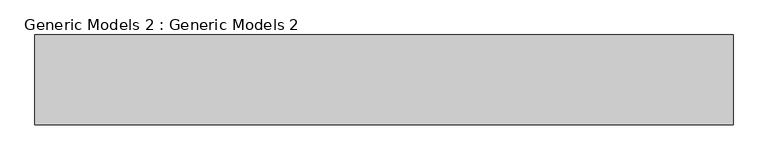
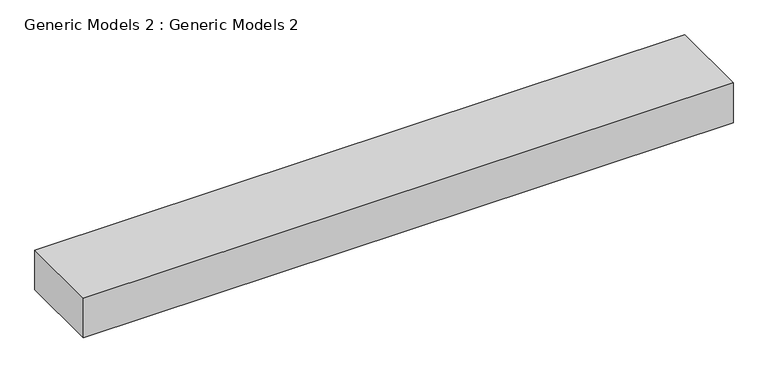
"""IFC4 building model written with IfcOpenShell, lengths in millimetres: proxy geometry, Generic Models 2 : Generic Models 2."""

from ifc_helpers import new_model, si_unit, frame, origin, place, context, project, spatial, polyline, outline, extrude, source, transform, mapped, element, save


def generic_models_2_generic_models_2_72429bd6(model_context):
    return source(origin(), model_context, "Body", "SweptSolid", [
        extrude(outline(polyline([(-12540.3371373, -3685.061407), (-14902.5371373, -3685.061407), (-14902.5371373, -3380.261407), (-12540.3371373, -3380.261407), (-12540.3371373, -3685.061407)])), frame((0.0, 0.0, 304.8), z_axis=(0.0, 0.0, 1.0), x_axis=(1.0, 0.0, 0.0)), (0.0, 0.0, 1.0), 152.4),
    ])


if __name__ == "__main__":
    model = new_model("IFC4")
    model_context = context("Model", 3, world=origin())
    ifc_project = project(units=[si_unit("LENGTHUNIT", "METRE", prefix="MILLI")], contexts=[model_context])
    site = spatial("IfcSite", under=ifc_project)
    building = spatial("IfcBuilding", under=site)
    placement = place(None, origin())
    generic_models_2_generic_models_2_shape = generic_models_2_generic_models_2_72429bd6(model_context)
    element("IfcBuildingElementProxy", 1, Name="Generic Models 2 : Generic Models 2", ObjectType="Generic Models 2 : Generic Models 2", at=placement, inside=building, context=model_context, shape_type="MappedRepresentation", body=[
        mapped(generic_models_2_generic_models_2_shape, transform((0.0, 0.0, 0.0), x_axis=(1.0, 0.0, 0.0), y_axis=(0.0, 1.0, 0.0), z_axis=(0.0, 0.0, 1.0))),
    ])
    save(model, "model.ifc")
